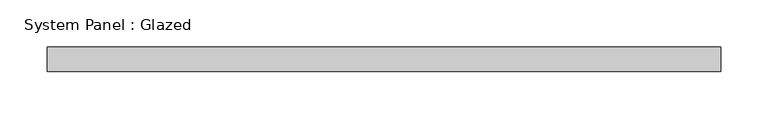
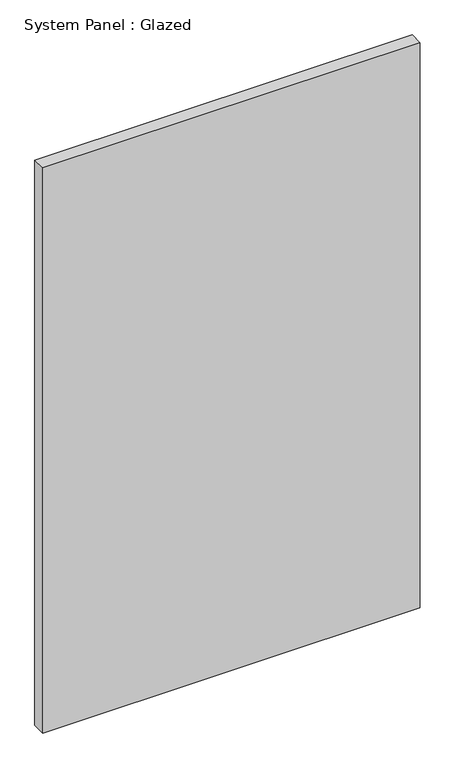
"""IFC4 building model written with IfcOpenShell, lengths in millimetres: plate geometry, System Panel : Glazed."""

from ifc_helpers import new_model, si_unit, origin, origin_with_axes, place, context, project, spatial, polyline, outline, extrude, source, transform, mapped, element, save


def system_panel_glazed_0ba8262e(model_context):
    return source(origin(), model_context, "Body", "SweptSolid", [
        extrude(outline(polyline([(354.5271, 19.05), (-354.5271, 19.05), (-354.5271, 44.45), (354.5271, 44.45), (354.5271, 19.05)])), origin_with_axes(), (0.0, 0.0, 1.0), 1121.8333333),
    ])


if __name__ == "__main__":
    model = new_model("IFC4")
    model_context = context("Model", 3, world=origin())
    ifc_project = project(units=[si_unit("LENGTHUNIT", "METRE", prefix="MILLI")], contexts=[model_context])
    site = spatial("IfcSite", under=ifc_project)
    building = spatial("IfcBuilding", under=site)
    placement = place(None, origin())
    system_panel_glazed_shape = system_panel_glazed_0ba8262e(model_context)
    element("IfcPlate", 1, ObjectType="System Panel : Glazed", at=placement, inside=building, context=model_context, shape_type="MappedRepresentation", body=[
        mapped(system_panel_glazed_shape, transform((0.0, 0.0, 0.0), x_axis=(1.0, 0.0, 0.0), y_axis=(0.0, 1.0, 0.0), z_axis=(0.0, 0.0, 1.0))),
    ])
    save(model, "model.ifc")

# Revit data of these elements
# Type "System Panel : Glazed"
#   Construction Type Id = "GSP4R"
#   Analytic Construction = "1/8 in Pilkington single glazing"
#   Visual Light Transmittance = 0.9
#   Solar Heat Gain Coefficient = 0.86
#   Heat Transfer Coefficient (U) = 1.18115 BTU/(h·ft²·°F)
#   Define Thermal Properties by = 1
# Element 1 (IfcPlate, "System Panel : Glazed")
#   Materials on its faces: "Glass"
# Materials
#   "Glass": class "Glass", colour RGB 0 128 192, transparency 0.75, Description = "Soda Lime Glass", Cost = 0
